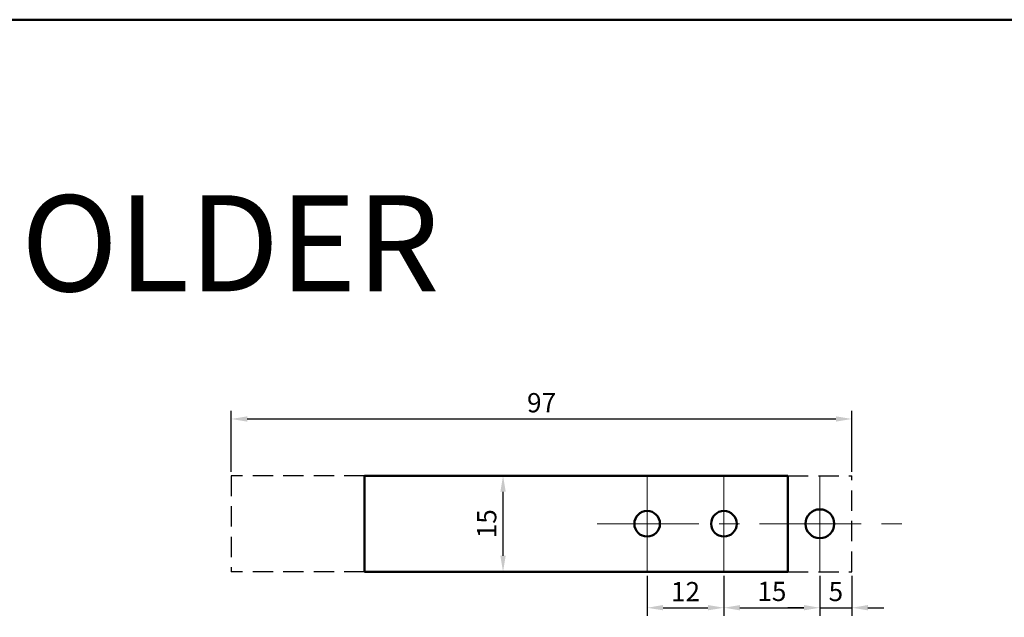
# Model space of a CAD drawing. Units: millimetres. Extents: x 77 to 718, y -35 to 313.
# Tile 6 of 7: x 379 to 533, y 220 to 313. Entities that reach past the tile are written whole.
import ezdxf

# ---------------------------------------------------------------- set-up
doc = ezdxf.new("R2010")
doc.units = ezdxf.units.MM
doc.header["$LTSCALE"] = 0.5
doc.linetypes.add('CENTER', pattern=[50.8, 31.75, -6.35, 6.35, -6.35])
doc.linetypes.add('HIDDEN', pattern=[9.525, 6.35, -3.175])
for name, color, linetype, lineweight in [('M-CNTR', 1, 'CENTER', 18), ('M-DIMS', 2, 'Continuous', 25), ('M-HIDN', 8, 'HIDDEN', 25), ('M-OUTL', 7, 'Continuous', 50), ('M-TEXT', 3, 'Continuous', 25)]:
    doc.layers.add(name, color=color, linetype=linetype, lineweight=lineweight)
doc.styles.get("Standard").update_dxf_attribs({"font": 'arial.ttf'})
doc.dimstyles.new('ISO-25', dxfattribs={"dimtxt": 3, "dimasz": 2.5, "dimexe": 1.25, "dimexo": 0.625, "dimtad": 1, "dimtxsty": 'Standard', "dimcen": 2.5, "dimadec": 0, "dimazin": 0, "dimtfac": 1, "dimtmove": 0, "dimatfit": 3, "dimfxl": 1, "dimarcsym": 0})

# ---------------------------------------------------------------- blocks, each defined once
blk = doc.blocks.new('*D88')
at = {"layer": 'Defpoints', "color": 0, "transparency": 16777216}
for p in [(477.28, 226.67), (489.28, 226.67), (489.28, 221.05)]:
    blk.add_point(p, dxfattribs=at)
at = {"layer": 'M-DIMS', "color": 0, "lineweight": -2, "transparency": 16777216}
for p, q in [((477.28, 226.04), (477.28, 219.8)), ((489.28, 226.04), (489.28, 219.8)), ((479.78, 221.05), (486.78, 221.05))]:
    blk.add_line(p, q, dxfattribs=at)
at = {"layer": 'M-DIMS', "color": 0, "transparency": 16777216}
for points in [[(479.78, 221.47), (479.78, 220.64), (477.28, 221.05)], [(486.78, 221.47), (486.78, 220.64), (489.28, 221.05)]]:
    blk.add_solid(points, dxfattribs=at)
at = {"layer": 'M-DIMS', "color": 0, "transparency": 16777216, "insert": (483.28, 223.18), "char_height": 3, "attachment_point": 5}
blk.add_mtext('12', dxfattribs=at)
blk = doc.blocks.new('*D89')
at = {"layer": 'Defpoints', "color": 0, "transparency": 16777216}
for p in [(489.28, 226.67), (504.28, 226.67), (504.28, 221.05)]:
    blk.add_point(p, dxfattribs=at)
at = {"layer": 'M-DIMS', "color": 0, "lineweight": -2, "transparency": 16777216}
for p, q in [((489.28, 226.04), (489.28, 219.8)), ((504.28, 226.04), (504.28, 219.8)), ((491.78, 221.05), (501.78, 221.05))]:
    blk.add_line(p, q, dxfattribs=at)
at = {"layer": 'M-DIMS', "color": 0, "transparency": 16777216}
for points in [[(491.78, 221.47), (491.78, 220.64), (489.28, 221.05)], [(501.78, 221.47), (501.78, 220.64), (504.28, 221.05)]]:
    blk.add_solid(points, dxfattribs=at)
at = {"layer": 'M-DIMS', "color": 0, "transparency": 16777216, "insert": (496.78, 223.21), "char_height": 3, "attachment_point": 5}
blk.add_mtext('15', dxfattribs=at)
blk = doc.blocks.new('*D90')
at = {"layer": 'Defpoints', "color": 0, "transparency": 16777216}
for p in [(504.28, 226.67), (509.28, 226.67), (509.28, 221.05)]:
    blk.add_point(p, dxfattribs=at)
at = {"layer": 'M-DIMS', "color": 0, "lineweight": -2, "transparency": 16777216}
for p, q in [((504.28, 226.04), (504.28, 219.8)), ((509.28, 226.04), (509.28, 219.8)), ((501.78, 221.05), (499.28, 221.05)), ((504.28, 221.05), (509.28, 221.05)), ((511.78, 221.05), (514.28, 221.05))]:
    blk.add_line(p, q, dxfattribs=at)
at = {"layer": 'M-DIMS', "color": 0, "transparency": 16777216}
for points in [[(501.78, 221.47), (501.78, 220.64), (504.28, 221.05)], [(511.78, 221.47), (511.78, 220.64), (509.28, 221.05)]]:
    blk.add_solid(points, dxfattribs=at)
at = {"layer": 'M-DIMS', "color": 0, "transparency": 16777216, "insert": (506.78, 223.2), "char_height": 3, "attachment_point": 5}
blk.add_mtext('5', dxfattribs=at)
blk = doc.blocks.new('*D91')
at = {"layer": 'Defpoints', "color": 0, "transparency": 16777216}
for p in [(509.28, 250.54), (412.28, 241.67), (509.28, 241.67)]:
    blk.add_point(p, dxfattribs=at)
at = {"layer": 'M-DIMS', "color": 0, "lineweight": -2, "transparency": 16777216}
for p, q in [((412.28, 242.29), (412.28, 251.79)), ((509.28, 242.29), (509.28, 251.79)), ((414.78, 250.54), (506.78, 250.54))]:
    blk.add_line(p, q, dxfattribs=at)
at = {"layer": 'M-DIMS', "color": 0, "transparency": 16777216}
for points in [[(414.78, 250.95), (414.78, 250.12), (412.28, 250.54)], [(506.78, 250.95), (506.78, 250.12), (509.28, 250.54)]]:
    blk.add_solid(points, dxfattribs=at)
at = {"layer": 'M-DIMS', "color": 0, "transparency": 16777216, "insert": (460.78, 252.69), "char_height": 3, "attachment_point": 5}
blk.add_mtext('97', dxfattribs=at)
blk = doc.blocks.new('*D92')
at = {"layer": 'Defpoints', "color": 0, "transparency": 16777216}
for p in [(449.16, 241.67), (454.76, 241.67), (458.26, 226.67)]:
    blk.add_point(p, dxfattribs=at)
at = {"layer": 'M-DIMS', "color": 0, "lineweight": -2, "transparency": 16777216}
for p, q in [((449.78, 241.67), (456.01, 241.67)), ((454.76, 229.17), (454.76, 239.17)), ((457.63, 226.67), (453.51, 226.67))]:
    blk.add_line(p, q, dxfattribs=at)
at = {"layer": 'M-DIMS', "color": 0, "transparency": 16777216}
for points in [[(454.34, 239.17), (455.18, 239.17), (454.76, 241.67)], [(454.34, 229.17), (455.18, 229.17), (454.76, 226.67)]]:
    blk.add_solid(points, dxfattribs=at)
at = {"layer": 'M-DIMS', "color": 0, "transparency": 16777216, "insert": (452.6, 234.17), "char_height": 3, "attachment_point": 5, "rotation": 90}
blk.add_mtext('15', dxfattribs=at)

msp = doc.modelspace()

# ---------------------------------------------------------------- linework, layer by layer
at = {"layer": 'M-CNTR'}
for p, q in [((477.284, 226.668), (477.284, 241.668)), ((489.284, 226.668), (489.284, 241.668)), ((504.284, 226.668), (504.284, 241.668)), ((469.471, 234.168), (517.108, 234.168))]:
    msp.add_line(p, q, dxfattribs=at)
at = {"layer": 'M-HIDN'}
for p, q in [((412.284, 241.668), (412.284, 226.668)), ((433.1, 241.668), (412.284, 241.668)), ((499.284, 241.668), (509.284, 241.668)), ((509.284, 226.668), (509.284, 241.668)), ((433.1, 226.668), (412.284, 226.668)), ((499.284, 226.668), (509.284, 226.668))]:
    msp.add_line(p, q, dxfattribs=at)
at = {"layer": 'M-OUTL'}
for p, q in [((433.1, 226.668), (433.1, 241.668)), ((499.284, 241.668), (433.1, 241.668)), ((499.284, 226.668), (499.284, 241.668)), ((433.1, 226.668), (499.284, 226.668))]:
    msp.add_line(p, q, dxfattribs=at)
at = {"layer": 'M-OUTL', "ltscale": 0.5}
msp.add_lwpolyline([(77.418, 312.912), (718.012, 312.912), (718.012, -34.898), (77.418, -34.898)], close=True, dxfattribs=at)
at = {"layer": 'M-OUTL'}
for centre, radius in [((477.284, 234.168), 2), ((489.284, 234.168), 2), ((504.284, 234.168), 2.25)]:
    msp.add_circle(centre, radius, dxfattribs=at)

# ---------------------------------------------------------------- texts
at = {"layer": 'M-TEXT', "ltscale": 0.5, "insert": (291.641, 285.482), "char_height": 15, "attachment_point": 1}
msp.add_mtext_dynamic_manual_height_columns('BRUSH HOLDER', width=204.65045, gutter_width=12.5, heights=[0], dxfattribs=at)

# ---------------------------------------------------------------- dimensions: what is measured, and where the dimension line sits
at = {"layer": 'M-DIMS'}
for base, p1, p2, picture, middle in [((509.284, 250.537), (412.284, 241.668), (509.284, 241.668), '*D91', (460.784, 252.694)), ((489.284, 221.053), (477.284, 226.668), (489.284, 226.668), '*D88', (483.284, 223.184)), ((504.284, 221.053), (489.284, 226.668), (504.284, 226.668), '*D89', (496.784, 223.209)), ((509.284, 221.053), (504.284, 226.668), (509.284, 226.668), '*D90', (506.784, 223.203))]:
    dim = msp.add_linear_dim(base=base, p1=p1, p2=p2, dimstyle='ISO-25', override={"dimclrd": 0, "dimclre": 0, "dimclrt": 0}, dxfattribs=at)
    dim.commit()
    dim.dimension.update_dxf_attribs({"geometry": picture, "text_midpoint": middle})
dim = msp.add_linear_dim(base=(454.761, 241.668), p1=(458.26, 226.668), p2=(449.159, 241.668), angle=90, dimstyle='ISO-25', override={"dimclrd": 0, "dimclre": 0, "dimclrt": 0}, dxfattribs=at)
dim.commit()
dim.dimension.update_dxf_attribs({"geometry": '*D92', "text_midpoint": (452.604, 234.168)})

doc.saveas('drawing.dxf')
